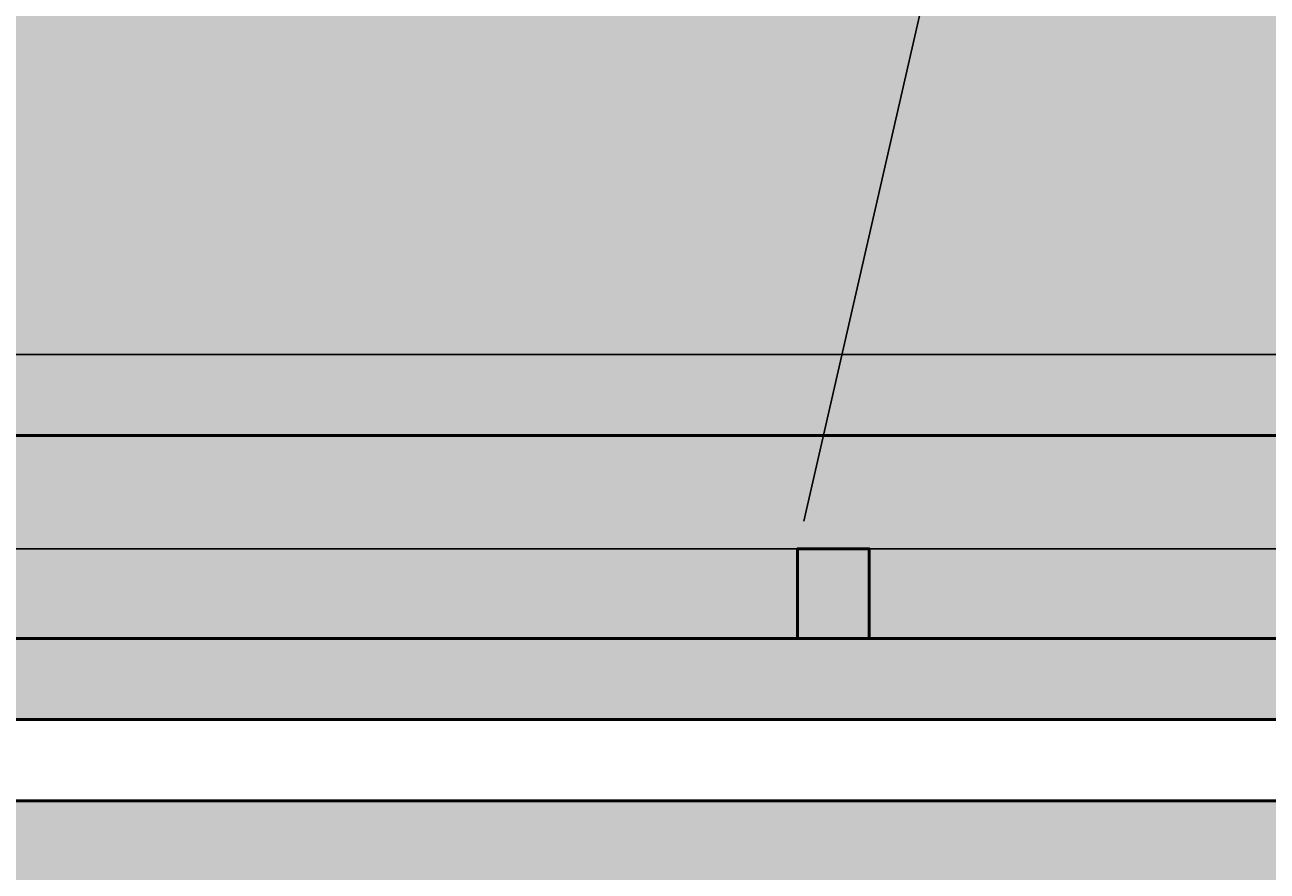
# Model space of a CAD drawing. Units: inches. Extents: x -12 to 334, y -10 to 186.
# Tile 45 of 77: x 152 to 182, y 90 to 111. Entities that reach past the tile are written whole.
import ezdxf
from ezdxf import colors
from ezdxf.entities.mleader import LeaderData, LeaderLine
from ezdxf.math import Vec2, Vec3

# ---------------------------------------------------------------- set-up
doc = ezdxf.new("R2010")
doc.units = ezdxf.units.IN
doc.header["$MEASUREMENT"] = 0
for name, color, linetype, lineweight in [('M-ANNO-TEXT', 3, 'Continuous', 25), ('M-DIMS', 2, 'Continuous', 18), ('M-EQPM', 7, 'Continuous', 50), ('M-EQPM-PATT', 8, 'Continuous', 18)]:
    doc.layers.add(name, color=color, linetype=linetype, lineweight=lineweight)
doc.styles.get("Standard").update_dxf_attribs({"font": 'arial.ttf'})
doc.dimstyles.get("Standard").update_dxf_attribs({"dimtxt": 0.18, "dimasz": 0.18, "dimexe": 0.18, "dimexo": 0.0625, "dimgap": 0.09, "dimtad": 0, "dimtih": 1, "dimtoh": 1, "dimdec": 4, "dimzin": 0, "dimdsep": 46, "dimtxsty": 'Standard', "dimcen": 0.09, "dimadec": 0, "dimazin": 0, "dimtfac": 1, "dimtdec": 4, "dimtofl": 0, "dimtmove": 0, "dimatfit": 3, "dimfxl": 1, "dimtolj": 1, "dimtzin": 0, "dimarcsym": 0})

# ---------------------------------------------------------------- blocks, each defined once
blk = doc.blocks.new('*D1')
at = {"layer": 'Defpoints', "color": 0, "transparency": 16777216}
for p in [(281.426, 91.899), (3.376, 80.692), (281.426, 14.304)]:
    blk.add_point(p, dxfattribs=at)
at = {"layer": 'M-DIMS', "color": 0, "lineweight": -2, "transparency": 16777216}
for p, q in [((281.426, 91.836), (281.426, 14.124)), ((3.376, 80.629), (3.376, 14.124)), ((3.556, 14.304), (141.935, 14.304)), ((281.246, 14.304), (142.867, 14.304))]:
    blk.add_line(p, q, dxfattribs=at)
at = {"layer": 'M-DIMS', "color": 0, "transparency": 16777216}
for points in [[(3.556, 14.334), (3.556, 14.274), (3.376, 14.304)], [(281.246, 14.334), (281.246, 14.274), (281.426, 14.304)]]:
    blk.add_solid(points, dxfattribs=at)
at = {"layer": 'M-DIMS', "color": 0, "transparency": 16777216, "insert": (142.401, 14.304), "char_height": 0.18, "attachment_point": 5}
blk.add_mtext('\\A1;278.05', dxfattribs=at)
blk = doc.blocks.new('*D17')
at = {"layer": 'Defpoints', "color": 0, "transparency": 16777216}
for p in [(106.177, 102.896), (105.892, 56.321), (295.976, 56.321)]:
    blk.add_point(p, dxfattribs=at)
at = {"layer": 'M-DIMS', "color": 0, "lineweight": -2, "transparency": 16777216}
for p, q in [((106.24, 102.896), (296.156, 102.896)), ((295.976, 102.716), (295.976, 79.79)), ((295.976, 56.501), (295.976, 79.426)), ((105.954, 56.321), (296.156, 56.321))]:
    blk.add_line(p, q, dxfattribs=at)
at = {"layer": 'M-DIMS', "color": 0, "transparency": 16777216}
for points in [[(295.946, 102.716), (296.006, 102.716), (295.976, 102.896)], [(295.946, 56.501), (296.006, 56.501), (295.976, 56.321)]]:
    blk.add_solid(points, dxfattribs=at)
at = {"layer": 'M-DIMS', "color": 0, "transparency": 16777216, "insert": (295.976, 79.608), "char_height": 0.18, "attachment_point": 5}
blk.add_mtext('\\A1;46.575', dxfattribs=at)
blk = doc.blocks.new('*D35')
at = {"layer": 'Defpoints', "color": 0, "transparency": 16777216}
for p in [(216.428, 98.108), (-11.174, 61.105), (216.428, 61.105)]:
    blk.add_point(p, dxfattribs=at)
at = {"layer": 'M-DIMS', "color": 0, "lineweight": -2, "transparency": 16777216}
for p, q in [((216.365, 98.108), (-11.354, 98.108)), ((-11.174, 97.928), (-11.174, 79.788)), ((-11.174, 61.285), (-11.174, 79.424)), ((216.365, 61.105), (-11.354, 61.105))]:
    blk.add_line(p, q, dxfattribs=at)
at = {"layer": 'M-DIMS', "color": 0, "transparency": 16777216}
for points in [[(-11.204, 97.928), (-11.144, 97.928), (-11.174, 98.108)], [(-11.204, 61.285), (-11.144, 61.285), (-11.174, 61.105)]]:
    blk.add_solid(points, dxfattribs=at)
at = {"layer": 'M-DIMS', "color": 0, "transparency": 16777216, "insert": (-11.174, 79.606), "char_height": 0.18, "attachment_point": 5}
blk.add_mtext('\\A1;37', dxfattribs=at)

msp = doc.modelspace()

# ---------------------------------------------------------------- hatches: boundary and pattern name
at = {"layer": 'M-EQPM-PATT', "transparency": 33554556}
h = msp.add_hatch(color=256, dxfattribs=at)
h.set_gradient(color1=(248, 206, 179), color2=(248, 206, 179), tint=1)
h.paths.add_polyline_path([(179.7818, 136.8871), (126.9567, 136.8871), (106.1771, 100.8958), (171.5458, 100.8958)])
h.paths.add_polyline_path([(268.3808, 136.9435), (214.0166, 136.9435), (214.0166, 154.8345), (196.3421, 154.8345), (196.3421, 136.8871), (179.7818, 136.8871), (171.5458, 100.8958), (231.7758, 100.8958, -0.4142136), (251.9801, 80.6915), (279.7263, 80.6915, 0.1631825)])
at = {"layer": 'M-EQPM-PATT'}
h = msp.add_hatch(color=256, dxfattribs=at)
h.set_gradient(color1=(205, 32, 39), color2=(205, 32, 39), tint=1)
h.paths.add_polyline_path([(64.5, 80.754), (64.5, 89.8963), (226.6083, 89.8963, -1), (226.6083, 69.6117), (64.5, 69.6117), (64.5, 78.754), (4.4744, 78.754, 0.384914), (23.5807, 61.4872), (37.1002, 61.4872), (37.1002, 33.6752), (53.1002, 33.6752), (53.1002, 61.4872), (64.5, 61.4872), (64.5, 63.6117), (226.6083, 63.6117, 1), (226.6083, 95.8963), (64.5, 95.8963), (64.5, 99.8958), (53.1002, 99.8958), (53.1002, 127.7078), (37.1002, 127.7078), (37.1002, 99.8958), (23.5807, 99.8958, 0.4132606), (4.3766, 80.754)])
h.paths.add_polyline_path([(64.5, 91.8963), (64.5, 93.8963), (226.6083, 93.8963, -1), (226.6083, 65.6117), (64.5, 65.6117), (64.5, 67.6117), (226.6083, 67.6117, 1), (226.6083, 91.8963)], flags=16)
h = msp.add_hatch(color=256, dxfattribs=at)
h.set_gradient(color1=(99, 100, 102), color2=(99, 100, 102), tint=1)
h.paths.add_polyline_path([(72.9244, 95.8963), (75.9244, 95.8963), (75.9244, 109.0583), (72.9244, 109.0583)])
h.paths.add_polyline_path([(72.9244, 50.4497), (75.9244, 50.4497), (75.9244, 63.6117), (72.9244, 63.6117)])
h.paths.add_polyline_path([(75.9244, 91.8963), (75.9244, 93.8963), (72.9244, 93.8963), (72.9244, 91.8963)])
h.paths.add_polyline_path([(75.9244, 65.6117), (75.9244, 67.6117), (72.9244, 67.6117), (72.9244, 65.6117)])
h.paths.add_polyline_path([(129.093, 69.6117), (130.8573, 69.6117), (130.8573, 89.8963), (129.093, 89.8963)])
h.paths.add_polyline_path([(129.093, 98.1081), (129.093, 95.8963), (130.8573, 95.8963), (130.8573, 98.1081)])
h.paths.add_polyline_path([(130.8573, 61.1045), (130.8573, 63.6117), (129.093, 63.6117), (129.093, 61.1045)])
h.paths.add_polyline_path([(170.9079, 69.6117), (172.6722, 69.6117), (172.6722, 89.8963), (170.9079, 89.8963)])
h.paths.add_polyline_path([(172.6722, 95.8963), (172.6722, 98.1081), (170.9079, 98.1081), (170.9079, 95.8963)])
h.paths.add_polyline_path([(170.9079, 61.1045), (172.6722, 61.1045), (172.6722, 63.6117), (170.9079, 63.6117)])
h.paths.add_polyline_path([(218.1922, 63.6117), (216.4278, 63.6117), (216.4278, 61.1045), (218.1922, 61.1045)])
h.paths.add_polyline_path([(216.4278, 69.6117), (218.1922, 69.6117), (218.1922, 89.8963), (216.4278, 89.8963)])
h.paths.add_polyline_path([(216.4278, 95.8963), (218.1922, 95.8963), (218.1922, 98.1081), (216.4278, 98.1081)])
h = msp.add_hatch(color=256, dxfattribs=at)
h.set_gradient(color1=(94, 103, 175), color2=(94, 103, 175), tint=1)
h.paths.add_polyline_path([(129.093, 89.8963), (86.8879, 89.8963), (86.8879, 69.6117), (129.093, 69.6117)], flags=17)
h.paths.add_polyline_path([(170.9079, 89.8963), (130.8573, 89.8963), (130.8573, 69.6117), (170.9079, 69.6117)], flags=17)
h.paths.add_polyline_path([(216.4278, 89.8963), (172.6722, 89.8963), (172.6722, 69.6117), (216.4278, 69.6117)], flags=17)
h.paths.add_polyline_path([(245.9354, 82.6969), (247.9354, 82.6969), (247.9354, 46.8541), (268.3808, 46.8541, 0.0998398), (279.7263, 80.6915), (251.9801, 80.6915, 0.4142136), (231.7758, 100.8958), (84.7229, 100.8958), (84.7229, 109.0583), (83.7229, 109.0583), (83.7229, 95.8963), (129.093, 95.8963), (129.093, 98.1081), (130.8573, 98.1081), (130.8573, 95.8963), (170.9079, 95.8963), (170.9079, 98.1081), (172.6722, 98.1081), (172.6722, 95.8963), (216.4278, 95.8963), (216.4278, 98.1081), (218.1922, 98.1081), (218.1922, 95.8963), (226.6083, 95.8963, -1), (226.6083, 63.6117), (218.1922, 63.6117), (218.1922, 61.1045), (216.4278, 61.1045), (216.4278, 63.6117), (172.6722, 63.6117), (172.6722, 61.1045), (170.9079, 61.1045), (170.9079, 63.6117), (130.8573, 63.6117), (130.8573, 61.1045), (129.093, 61.1045), (129.093, 63.6117), (87.8879, 63.6117), (87.8879, 56.3205), (105.8919, 56.3205), (105.8919, 28.8541), (115.8919, 28.8541), (115.8919, 46.8541), (222.5761, 46.8541), (222.5761, 30.8541), (232.5761, 30.8541), (232.5761, 46.8541), (245.9354, 46.8541)])
h.paths.add_polyline_path([(86.8879, 89.8963), (75.9244, 89.8963), (75.9244, 69.6117), (86.8879, 69.6117)])
h.paths.add_polyline_path([(83.7229, 109.0583), (75.9244, 109.0583), (75.9244, 95.8963), (83.7229, 95.8963)])
h.paths.add_polyline_path([(226.6083, 89.8963), (218.1922, 89.8963), (218.1922, 69.6117), (226.6083, 69.6117, 1)], flags=17)
h = msp.add_hatch(color=256, dxfattribs=at)
h.set_gradient(color1=(0, 0, 255), color2=(0, 0, 255), tint=1)
h.paths.add_polyline_path([(84.7229, 100.8958), (84.7229, 109.0583), (83.7229, 109.0583), (83.7229, 95.8963), (129.093, 95.8963), (129.093, 98.1081), (130.8573, 98.1081), (130.8573, 95.8963), (170.9079, 95.8963), (170.9079, 98.1081), (172.6722, 98.1081), (172.6722, 95.8963), (216.4278, 95.8963), (216.4278, 98.1081), (218.1922, 98.1081), (218.1922, 95.8963), (226.6083, 95.8963, -1), (226.6083, 63.6117), (218.1922, 63.6117), (218.1922, 61.1045), (216.4278, 61.1045), (216.4278, 63.6117), (172.6722, 63.6117), (172.6722, 61.1045), (170.9079, 61.1045), (170.9079, 63.6117), (130.8573, 63.6117), (130.8573, 61.1045), (129.093, 61.1045), (129.093, 63.6117), (87.8879, 63.6117), (87.8879, 56.3205), (105.8919, 56.3205), (105.8919, 28.8541), (115.8919, 28.8541), (115.8919, 46.8541), (222.5761, 46.8541), (222.5761, 30.8541), (232.5761, 30.8541), (232.5761, 46.8541), (245.9354, 46.8541), (245.9354, 82.6969), (247.9354, 82.6969), (247.9354, 46.8541), (268.3808, 46.8541, 0.0998398), (279.7263, 80.6915), (251.9801, 80.6915, 0.4142136), (231.7758, 100.8958)])

# ---------------------------------------------------------------- linework, layer by layer
at = {"layer": 'M-EQPM'}
for points in [[(84.7229, 100.8958), (231.7758, 100.8958)], [(170.9079, 95.8963), (170.9079, 98.1081), (172.6722, 98.1081), (172.6722, 95.8963)]]:
    msp.add_lwpolyline(points, dxfattribs=at)
for points in [[(64.5, 63.6117), (226.6083, 63.6117, 1), (226.6083, 95.8963), (64.5, 95.8963)], [(64.5, 65.6117), (226.6083, 65.6117, 1), (226.6083, 93.8963), (64.5, 93.8963)], [(64.5, 67.6117), (226.6083, 67.6117, 1), (226.6083, 91.8963), (64.5, 91.8963)]]:
    msp.add_lwpolyline(points, format="xyb", dxfattribs=at)

# ---------------------------------------------------------------- dimensions: what is measured, and where the dimension line sits
at = {"layer": 'M-DIMS'}
for base, p1, p2, override, picture, middle in [((295.9756, 56.3205), (106.1771, 102.8958), (105.8919, 56.3205), {"dimdec": 3, "dimlfac": 1, "dimrnd": 0, "dimzin": 0, "dimdsep": 46, "dimlunit": 2}, '*D17', (295.9756, 79.6082)), ((-11.1736, 61.1045), (216.4278, 98.1081), (216.4278, 61.1045), {"dimdec": 0, "dimlfac": 1, "dimrnd": 0, "dimzin": 0, "dimdsep": 46, "dimlunit": 2}, '*D35', (-11.1735, 79.6063))]:
    dim = msp.add_linear_dim(base=base, p1=p1, p2=p2, angle=90, dimstyle='Standard', override=override, dxfattribs=at)
    dim.commit()
    dim.dimension.update_dxf_attribs({"geometry": picture, "text_midpoint": middle})
dim = msp.add_linear_dim(base=(281.4256, 14.3041), p1=(3.3765, 80.6915), p2=(281.4256, 91.8988), dimstyle='Standard', override={"dimdec": 2, "dimlfac": 1, "dimrnd": 0, "dimzin": 0, "dimdsep": 46, "dimlunit": 2}, dxfattribs=at)
dim.commit()
dim.dimension.update_dxf_attribs({"geometry": '*D1', "text_midpoint": (142.401, 14.3041)})

# ---------------------------------------------------------------- leaders
at = {"layer": 'M-ANNO-TEXT'}
ml = msp.add_multileader_mtext('Standard', dxfattribs=at)
ml.set_content('Tube supports', color=256)
ml.set_leader_properties()
ml.build(insert=Vec2(0, 0))
ml.multileader.update_dxf_attribs({"dogleg_length": 0.36, "arrow_head_size": 0.7})
ctx = ml.context
ctx.base_point, ctx.arrow_head_size, ctx.landing_gap_size, ctx.plane_origin = Vec3(129.4363, 148.4609), 0.7, 0.09, Vec3(117.375, 151.6517)
ctx.text_align_type = 2
notes = []
notes.append((ctx, [(1, (1, 1, 0), (182.4302, 148.4609), (-1, 0), 17.4388, [(0, [(170.9079, 98.1081)], 0, [])])]))
ctx.mtext.insert, ctx.mtext.alignment, ctx.mtext.flow_direction = Vec3(164.9015, 151.0162), 3, 5
for ctx, leaders in notes:
    for number, flags, end, landing, length, lines in leaders:
        leader = LeaderData()
        leader.index, (leader.has_last_leader_line, leader.has_dogleg_vector, leader.attachment_direction) = number, flags
        leader.last_leader_point, leader.dogleg_vector, leader.dogleg_length = Vec3(end), Vec3(landing), length
        for number, points, colour, breaks in lines:
            line = LeaderLine()
            line.index, line.vertices, line.color, line.breaks = number, Vec3.list(points), colors.encode_raw_color(colour), breaks
            leader.lines.append(line)
        ctx.leaders.append(leader)

doc.saveas('drawing.dxf')
